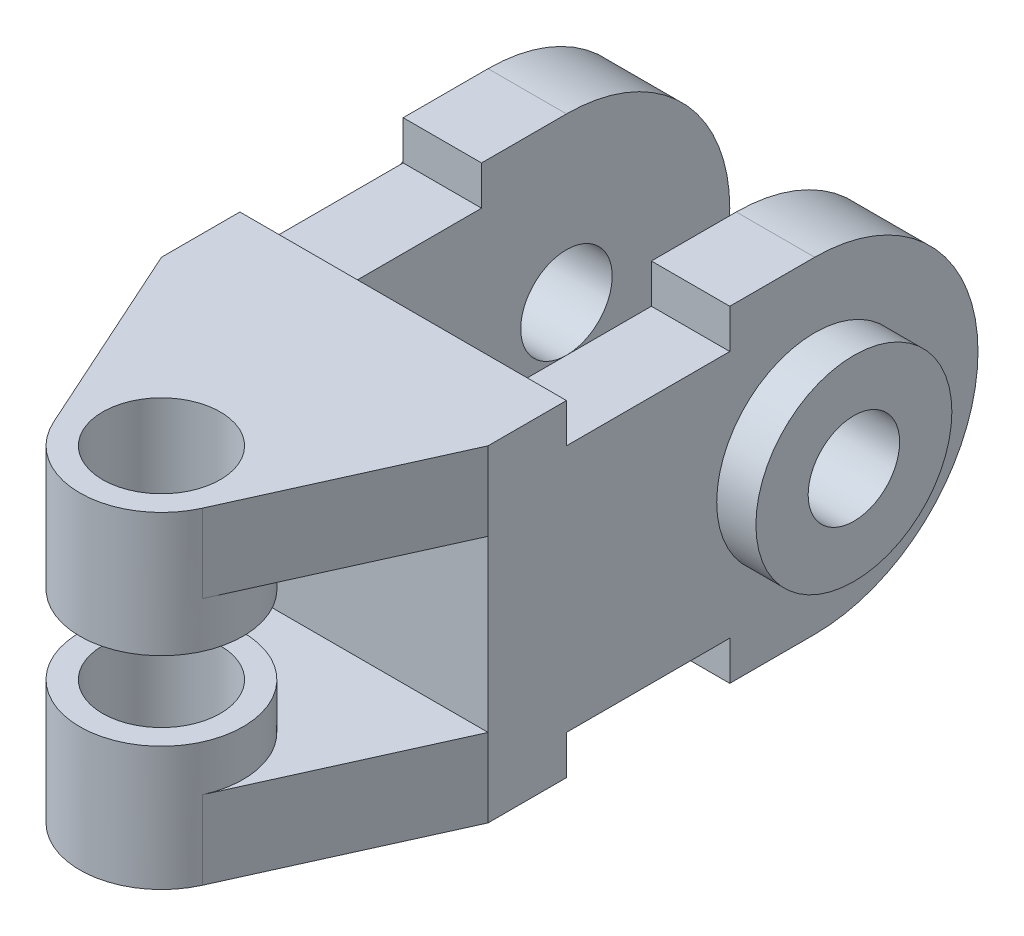
ISO-10303-21;
HEADER;
FILE_DESCRIPTION(('STEP AP214'),'2;1');
FILE_NAME('part.step','',(''),(''),'','','');
FILE_SCHEMA(('AUTOMOTIVE_DESIGN { 1 0 10303 214 1 1 1 1 }'));
ENDSEC;
DATA;
#1=APPLICATION_CONTEXT('core data for automotive mechanical design processes');
#2=APPLICATION_PROTOCOL_DEFINITION('international standard','automotive_design',2000,#1);
#3=PRODUCT_CONTEXT('',#1,'mechanical');
#4=PRODUCT('Part','Part','',(#3));
#5=PRODUCT_RELATED_PRODUCT_CATEGORY('part','',(#4));
#6=PRODUCT_DEFINITION_FORMATION('','',#4);
#7=PRODUCT_DEFINITION_CONTEXT('part definition',#1,'design');
#8=PRODUCT_DEFINITION('design','',#6,#7);
#9=PRODUCT_DEFINITION_SHAPE('','',#8);
#10=(LENGTH_UNIT() NAMED_UNIT(*) SI_UNIT(.MILLI.,.METRE.));
#11=(NAMED_UNIT(*) PLANE_ANGLE_UNIT() SI_UNIT($,.RADIAN.));
#12=(NAMED_UNIT(*) SI_UNIT($,.STERADIAN.) SOLID_ANGLE_UNIT());
#13=UNCERTAINTY_MEASURE_WITH_UNIT(LENGTH_MEASURE(1.E-05),#10,'distance_accuracy_value','');
#14=(GEOMETRIC_REPRESENTATION_CONTEXT(3) GLOBAL_UNCERTAINTY_ASSIGNED_CONTEXT((#13)) GLOBAL_UNIT_ASSIGNED_CONTEXT((#10,
#11,#12)) REPRESENTATION_CONTEXT('',''));
#15=CARTESIAN_POINT('',(0.,0.,0.));
#16=DIRECTION('',(0.,0.,1.));
#17=DIRECTION('',(1.,0.,0.));
#18=AXIS2_PLACEMENT_3D('',#15,#16,#17);
#19=CARTESIAN_POINT('',(0.,12.,0.));
#20=DIRECTION('',(0.,-1.,0.));
#21=DIRECTION('',(0.,0.,-1.));
#22=AXIS2_PLACEMENT_3D('',#19,#20,#21);
#23=PLANE('',#22);
#24=CARTESIAN_POINT('',(-13.,12.,25.));
#25=DIRECTION('',(0.,1.,0.));
#26=DIRECTION('',(0.,0.,1.));
#27=AXIS2_PLACEMENT_3D('',#24,#25,#26);
#28=CIRCLE('',#27,12.5);
#29=CARTESIAN_POINT('',(-1.60702715292317,12.,30.1429728470769));
#30=VERTEX_POINT('',#29);
#31=CARTESIAN_POINT('',(-24.3929728470769,12.,30.1429728470769));
#32=VERTEX_POINT('',#31);
#33=EDGE_CURVE('E226',#30,#32,#28,.T.);
#34=ORIENTED_EDGE('',*,*,#33,.F.);
#35=DIRECTION('',(0.411437827766148,0.,-0.911437827766148));
#36=VECTOR('',#35,1.);
#37=CARTESIAN_POINT('',(9.96862696659688,12.,4.5));
#38=LINE('',#37,#36);
#39=CARTESIAN_POINT('',(12.,12.,0.));
#40=VERTEX_POINT('',#39);
#41=EDGE_CURVE('E234',#30,#40,#38,.T.);
#42=ORIENTED_EDGE('',*,*,#41,.T.);
#43=DIRECTION('',(-1.,0.,0.));
#44=VECTOR('',#43,1.);
#45=CARTESIAN_POINT('',(0.,12.,0.));
#46=LINE('',#45,#44);
#47=CARTESIAN_POINT('',(-38.,12.,0.));
#48=VERTEX_POINT('',#47);
#49=EDGE_CURVE('E233',#40,#48,#46,.T.);
#50=ORIENTED_EDGE('',*,*,#49,.T.);
#51=DIRECTION('',(0.411437827766148,0.,0.911437827766148));
#52=VECTOR('',#51,1.);
#53=CARTESIAN_POINT('',(-31.5673187275568,12.,14.25));
#54=LINE('',#53,#52);
#55=EDGE_CURVE('E217',#48,#32,#54,.T.);
#56=ORIENTED_EDGE('',*,*,#55,.T.);
#57=EDGE_LOOP('',(#34,#42,#50,#56));
#58=FACE_BOUND('',#57,.T.);
#59=ADVANCED_FACE('F41',(#58),#23,.F.);
#60=CARTESIAN_POINT('',(12.,0.,0.));
#61=DIRECTION('',(0.,0.,-1.));
#62=DIRECTION('',(-1.,0.,0.));
#63=AXIS2_PLACEMENT_3D('',#60,#61,#62);
#64=PLANE('',#63);
#65=ORIENTED_EDGE('',*,*,#49,.F.);
#66=DIRECTION('',(0.,-1.,0.));
#67=VECTOR('',#66,1.);
#68=CARTESIAN_POINT('',(12.,0.,0.));
#69=LINE('',#68,#67);
#70=CARTESIAN_POINT('',(12.,38.,0.));
#71=VERTEX_POINT('',#70);
#72=EDGE_CURVE('E403',#71,#40,#69,.T.);
#73=ORIENTED_EDGE('',*,*,#72,.F.);
#74=DIRECTION('',(-1.,0.,0.));
#75=VECTOR('',#74,1.);
#76=CARTESIAN_POINT('',(-38.,38.,0.));
#77=LINE('',#76,#75);
#78=CARTESIAN_POINT('',(-38.,38.,0.));
#79=VERTEX_POINT('',#78);
#80=EDGE_CURVE('E267',#71,#79,#77,.T.);
#81=ORIENTED_EDGE('',*,*,#80,.T.);
#82=DIRECTION('',(0.,-1.,0.));
#83=VECTOR('',#82,1.);
#84=CARTESIAN_POINT('',(-38.,50.,0.));
#85=LINE('',#84,#83);
#86=EDGE_CURVE('E355',#79,#48,#85,.T.);
#87=ORIENTED_EDGE('',*,*,#86,.T.);
#88=EDGE_LOOP('',(#65,#73,#81,#87));
#89=FACE_BOUND('',#88,.T.);
#90=ADVANCED_FACE('F481',(#89),#64,.F.);
#91=CARTESIAN_POINT('',(-38.,50.,-12.));
#92=DIRECTION('',(-1.,0.,0.));
#93=DIRECTION('',(0.,0.,1.));
#94=AXIS2_PLACEMENT_3D('',#91,#92,#93);
#95=PLANE('',#94);
#96=CARTESIAN_POINT('',(-38.,50.,0.));
#97=VERTEX_POINT('',#96);
#98=EDGE_CURVE('E375',#97,#79,#85,.T.);
#99=ORIENTED_EDGE('',*,*,#98,.F.);
#100=DIRECTION('',(0.,0.,1.));
#101=VECTOR('',#100,1.);
#102=CARTESIAN_POINT('',(-38.,50.,-12.));
#103=LINE('',#102,#101);
#104=CARTESIAN_POINT('',(-38.,50.,-12.));
#105=VERTEX_POINT('',#104);
#106=EDGE_CURVE('E367',#105,#97,#103,.T.);
#107=ORIENTED_EDGE('',*,*,#106,.F.);
#108=DIRECTION('',(0.,-1.,0.));
#109=VECTOR('',#108,1.);
#110=CARTESIAN_POINT('',(-38.,50.,-12.));
#111=LINE('',#110,#109);
#112=CARTESIAN_POINT('',(-38.,44.,-12.));
#113=VERTEX_POINT('',#112);
#114=EDGE_CURVE('E370',#105,#113,#111,.T.);
#115=ORIENTED_EDGE('',*,*,#114,.T.);
#116=DIRECTION('',(0.,0.,-1.));
#117=VECTOR('',#116,1.);
#118=CARTESIAN_POINT('',(-38.,44.,-12.));
#119=LINE('',#118,#117);
#120=CARTESIAN_POINT('',(-38.,44.,-37.));
#121=VERTEX_POINT('',#120);
#122=EDGE_CURVE('E307',#113,#121,#119,.T.);
#123=ORIENTED_EDGE('',*,*,#122,.T.);
#124=DIRECTION('',(0.,1.,0.));
#125=VECTOR('',#124,1.);
#126=CARTESIAN_POINT('',(-38.,44.,-37.));
#127=LINE('',#126,#125);
#128=CARTESIAN_POINT('',(-38.,50.,-37.));
#129=VERTEX_POINT('',#128);
#130=EDGE_CURVE('E333',#121,#129,#127,.T.);
#131=ORIENTED_EDGE('',*,*,#130,.T.);
#132=DIRECTION('',(0.,0.,-1.));
#133=VECTOR('',#132,1.);
#134=CARTESIAN_POINT('',(-38.,50.,-37.));
#135=LINE('',#134,#133);
#136=CARTESIAN_POINT('',(-38.,50.,-50.));
#137=VERTEX_POINT('',#136);
#138=EDGE_CURVE('E338',#129,#137,#135,.T.);
#139=ORIENTED_EDGE('',*,*,#138,.T.);
#140=CARTESIAN_POINT('',(-38.,25.,-50.));
#141=DIRECTION('',(-1.,0.,0.));
#142=DIRECTION('',(0.,0.,1.));
#143=AXIS2_PLACEMENT_3D('',#140,#141,#142);
#144=CIRCLE('',#143,25.);
#145=CARTESIAN_POINT('',(-38.,0.,-50.));
#146=VERTEX_POINT('',#145);
#147=EDGE_CURVE('E342',#137,#146,#144,.T.);
#148=ORIENTED_EDGE('',*,*,#147,.T.);
#149=DIRECTION('',(0.,0.,1.));
#150=VECTOR('',#149,1.);
#151=CARTESIAN_POINT('',(-38.,0.,-37.));
#152=LINE('',#151,#150);
#153=CARTESIAN_POINT('',(-38.,0.,-37.));
#154=VERTEX_POINT('',#153);
#155=EDGE_CURVE('E344',#146,#154,#152,.T.);
#156=ORIENTED_EDGE('',*,*,#155,.T.);
#157=DIRECTION('',(0.,1.,0.));
#158=VECTOR('',#157,1.);
#159=CARTESIAN_POINT('',(-38.,6.,-37.));
#160=LINE('',#159,#158);
#161=CARTESIAN_POINT('',(-38.,6.,-37.));
#162=VERTEX_POINT('',#161);
#163=EDGE_CURVE('E350',#154,#162,#160,.T.);
#164=ORIENTED_EDGE('',*,*,#163,.T.);
#165=DIRECTION('',(0.,0.,1.));
#166=VECTOR('',#165,1.);
#167=CARTESIAN_POINT('',(-38.,6.,-12.));
#168=LINE('',#167,#166);
#169=CARTESIAN_POINT('',(-38.,6.,-12.));
#170=VERTEX_POINT('',#169);
#171=EDGE_CURVE('E64',#162,#170,#168,.T.);
#172=ORIENTED_EDGE('',*,*,#171,.T.);
#173=CARTESIAN_POINT('',(-38.,0.,-12.));
#174=VERTEX_POINT('',#173);
#175=EDGE_CURVE('E371',#170,#174,#111,.T.);
#176=ORIENTED_EDGE('',*,*,#175,.T.);
#177=DIRECTION('',(0.,0.,1.));
#178=VECTOR('',#177,1.);
#179=CARTESIAN_POINT('',(-38.,0.,-12.));
#180=LINE('',#179,#178);
#181=CARTESIAN_POINT('',(-38.,0.,0.));
#182=VERTEX_POINT('',#181);
#183=EDGE_CURVE('E372',#174,#182,#180,.T.);
#184=ORIENTED_EDGE('',*,*,#183,.T.);
#185=DIRECTION('',(0.,-1.,0.));
#186=VECTOR('',#185,1.);
#187=CARTESIAN_POINT('',(-38.,12.,0.));
#188=LINE('',#187,#186);
#189=EDGE_CURVE('E227',#48,#182,#188,.T.);
#190=ORIENTED_EDGE('',*,*,#189,.F.);
#191=ORIENTED_EDGE('',*,*,#86,.F.);
#192=EDGE_LOOP('',(#99,#107,#115,#123,#131,#139,#148,#156,#164,#172,#176,#184,#190,#191));
#193=FACE_BOUND('',#192,.T.);
#194=CARTESIAN_POINT('',(-38.,25.,-50.));
#195=DIRECTION('',(-1.,0.,0.));
#196=DIRECTION('',(0.,0.,1.));
#197=AXIS2_PLACEMENT_3D('',#194,#195,#196);
#198=CIRCLE('',#197,15.);
#199=CARTESIAN_POINT('',(-38.,25.,-35.));
#200=VERTEX_POINT('',#199);
#201=EDGE_CURVE('E292',#200,#200,#198,.T.);
#202=ORIENTED_EDGE('',*,*,#201,.F.);
#203=EDGE_LOOP('',(#202));
#204=FACE_BOUND('',#203,.T.);
#205=ADVANCED_FACE('F488',(#193,#204),#95,.T.);
#206=CARTESIAN_POINT('',(12.,0.,-12.));
#207=DIRECTION('',(0.,1.,0.));
#208=DIRECTION('',(0.,0.,1.));
#209=AXIS2_PLACEMENT_3D('',#206,#207,#208);
#210=PLANE('',#209);
#211=DIRECTION('',(0.,0.,-1.));
#212=VECTOR('',#211,1.);
#213=CARTESIAN_POINT('',(12.,0.,-12.));
#214=LINE('',#213,#212);
#215=CARTESIAN_POINT('',(12.,0.,0.));
#216=VERTEX_POINT('',#215);
#217=CARTESIAN_POINT('',(12.,0.,-12.));
#218=VERTEX_POINT('',#217);
#219=EDGE_CURVE('E379',#216,#218,#214,.T.);
#220=ORIENTED_EDGE('',*,*,#219,.F.);
#221=DIRECTION('',(0.411437827766148,0.,-0.911437827766148));
#222=VECTOR('',#221,1.);
#223=CARTESIAN_POINT('',(9.96862696659688,0.,4.5));
#224=LINE('',#223,#222);
#225=CARTESIAN_POINT('',(-1.60702715292317,0.,30.1429728470769));
#226=VERTEX_POINT('',#225);
#227=EDGE_CURVE('E243',#226,#216,#224,.T.);
#228=ORIENTED_EDGE('',*,*,#227,.F.);
#229=CARTESIAN_POINT('',(-13.,0.,25.));
#230=DIRECTION('',(0.,-1.,0.));
#231=DIRECTION('',(0.,0.,-1.));
#232=AXIS2_PLACEMENT_3D('',#229,#230,#231);
#233=CIRCLE('',#232,12.5);
#234=CARTESIAN_POINT('',(-24.3929728470768,0.,30.1429728470769));
#235=VERTEX_POINT('',#234);
#236=EDGE_CURVE('E252',#226,#235,#233,.T.);
#237=ORIENTED_EDGE('',*,*,#236,.T.);
#238=DIRECTION('',(0.411437827766148,0.,0.911437827766148));
#239=VECTOR('',#238,1.);
#240=CARTESIAN_POINT('',(-31.5673187275568,0.,14.25));
#241=LINE('',#240,#239);
#242=EDGE_CURVE('E222',#182,#235,#241,.T.);
#243=ORIENTED_EDGE('',*,*,#242,.F.);
#244=ORIENTED_EDGE('',*,*,#183,.F.);
#245=DIRECTION('',(-1.,0.,0.));
#246=VECTOR('',#245,1.);
#247=CARTESIAN_POINT('',(12.,0.,-12.));
#248=LINE('',#247,#246);
#249=EDGE_CURVE('E448',#218,#174,#248,.T.);
#250=ORIENTED_EDGE('',*,*,#249,.F.);
#251=EDGE_LOOP('',(#220,#228,#237,#243,#244,#250));
#252=FACE_BOUND('',#251,.T.);
#253=CARTESIAN_POINT('',(-13.,0.,25.));
#254=DIRECTION('',(0.,-1.,0.));
#255=DIRECTION('',(0.,0.,-1.));
#256=AXIS2_PLACEMENT_3D('',#253,#254,#255);
#257=CIRCLE('',#256,9.);
#258=CARTESIAN_POINT('',(-13.,0.,16.));
#259=VERTEX_POINT('',#258);
#260=EDGE_CURVE('E248',#259,#259,#257,.T.);
#261=ORIENTED_EDGE('',*,*,#260,.F.);
#262=EDGE_LOOP('',(#261));
#263=FACE_BOUND('',#262,.T.);
#264=ADVANCED_FACE('F43',(#252,#263),#210,.F.);
#265=CARTESIAN_POINT('',(12.,6.,-37.));
#266=DIRECTION('',(0.,1.,0.));
#267=DIRECTION('',(0.,0.,1.));
#268=AXIS2_PLACEMENT_3D('',#265,#266,#267);
#269=PLANE('',#268);
#270=DIRECTION('',(0.,0.,-1.));
#271=VECTOR('',#270,1.);
#272=CARTESIAN_POINT('',(0.,6.,-37.));
#273=LINE('',#272,#271);
#274=CARTESIAN_POINT('',(0.,6.,-12.));
#275=VERTEX_POINT('',#274);
#276=CARTESIAN_POINT('',(0.,6.,-37.));
#277=VERTEX_POINT('',#276);
#278=EDGE_CURVE('E380',#275,#277,#273,.T.);
#279=ORIENTED_EDGE('',*,*,#278,.T.);
#280=DIRECTION('',(-1.,0.,0.));
#281=VECTOR('',#280,1.);
#282=CARTESIAN_POINT('',(12.,6.,-37.));
#283=LINE('',#282,#281);
#284=CARTESIAN_POINT('',(12.,6.,-37.));
#285=VERTEX_POINT('',#284);
#286=EDGE_CURVE('E445',#285,#277,#283,.T.);
#287=ORIENTED_EDGE('',*,*,#286,.F.);
#288=DIRECTION('',(0.,0.,-1.));
#289=VECTOR('',#288,1.);
#290=CARTESIAN_POINT('',(12.,6.,-37.));
#291=LINE('',#290,#289);
#292=CARTESIAN_POINT('',(12.,6.,-12.));
#293=VERTEX_POINT('',#292);
#294=EDGE_CURVE('E387',#293,#285,#291,.T.);
#295=ORIENTED_EDGE('',*,*,#294,.F.);
#296=DIRECTION('',(-1.,0.,0.));
#297=VECTOR('',#296,1.);
#298=CARTESIAN_POINT('',(12.,6.,-12.));
#299=LINE('',#298,#297);
#300=EDGE_CURVE('E443',#293,#275,#299,.T.);
#301=ORIENTED_EDGE('',*,*,#300,.T.);
#302=EDGE_LOOP('',(#279,#287,#295,#301));
#303=FACE_BOUND('',#302,.T.);
#304=ADVANCED_FACE('F591',(#303),#269,.F.);
#305=CARTESIAN_POINT('',(12.,0.,-37.));
#306=DIRECTION('',(0.,0.,-1.));
#307=DIRECTION('',(-1.,0.,0.));
#308=AXIS2_PLACEMENT_3D('',#305,#306,#307);
#309=PLANE('',#308);
#310=DIRECTION('',(0.,-1.,0.));
#311=VECTOR('',#310,1.);
#312=CARTESIAN_POINT('',(0.,0.,-37.));
#313=LINE('',#312,#311);
#314=CARTESIAN_POINT('',(0.,0.,-37.));
#315=VERTEX_POINT('',#314);
#316=EDGE_CURVE('E412',#277,#315,#313,.T.);
#317=ORIENTED_EDGE('',*,*,#316,.T.);
#318=DIRECTION('',(-1.,0.,0.));
#319=VECTOR('',#318,1.);
#320=CARTESIAN_POINT('',(12.,0.,-37.));
#321=LINE('',#320,#319);
#322=CARTESIAN_POINT('',(12.,0.,-37.));
#323=VERTEX_POINT('',#322);
#324=EDGE_CURVE('E438',#323,#315,#321,.T.);
#325=ORIENTED_EDGE('',*,*,#324,.F.);
#326=DIRECTION('',(0.,-1.,0.));
#327=VECTOR('',#326,1.);
#328=CARTESIAN_POINT('',(12.,0.,-37.));
#329=LINE('',#328,#327);
#330=EDGE_CURVE('E389',#285,#323,#329,.T.);
#331=ORIENTED_EDGE('',*,*,#330,.F.);
#332=ORIENTED_EDGE('',*,*,#286,.T.);
#333=EDGE_LOOP('',(#317,#325,#331,#332));
#334=FACE_BOUND('',#333,.T.);
#335=ADVANCED_FACE('F596',(#334),#309,.F.);
#336=CARTESIAN_POINT('',(12.,0.,-50.));
#337=DIRECTION('',(0.,1.,0.));
#338=DIRECTION('',(0.,0.,1.));
#339=AXIS2_PLACEMENT_3D('',#336,#337,#338);
#340=PLANE('',#339);
#341=DIRECTION('',(0.,0.,-1.));
#342=VECTOR('',#341,1.);
#343=CARTESIAN_POINT('',(0.,0.,-50.));
#344=LINE('',#343,#342);
#345=CARTESIAN_POINT('',(0.,0.,-50.));
#346=VERTEX_POINT('',#345);
#347=EDGE_CURVE('E413',#315,#346,#344,.T.);
#348=ORIENTED_EDGE('',*,*,#347,.T.);
#349=DIRECTION('',(-1.,0.,0.));
#350=VECTOR('',#349,1.);
#351=CARTESIAN_POINT('',(12.,0.,-50.));
#352=LINE('',#351,#350);
#353=CARTESIAN_POINT('',(12.,0.,-50.));
#354=VERTEX_POINT('',#353);
#355=EDGE_CURVE('E436',#354,#346,#352,.T.);
#356=ORIENTED_EDGE('',*,*,#355,.F.);
#357=DIRECTION('',(0.,0.,-1.));
#358=VECTOR('',#357,1.);
#359=CARTESIAN_POINT('',(12.,0.,-50.));
#360=LINE('',#359,#358);
#361=EDGE_CURVE('E388',#323,#354,#360,.T.);
#362=ORIENTED_EDGE('',*,*,#361,.F.);
#363=ORIENTED_EDGE('',*,*,#324,.T.);
#364=EDGE_LOOP('',(#348,#356,#362,#363));
#365=FACE_BOUND('',#364,.T.);
#366=ADVANCED_FACE('F605',(#365),#340,.F.);
#367=CARTESIAN_POINT('',(12.,25.,-50.));
#368=DIRECTION('',(-1.,0.,0.));
#369=DIRECTION('',(0.,0.,1.));
#370=AXIS2_PLACEMENT_3D('',#367,#368,#369);
#371=CYLINDRICAL_SURFACE('',#370,25.);
#372=CARTESIAN_POINT('',(0.,25.,-50.));
#373=DIRECTION('',(1.,0.,0.));
#374=DIRECTION('',(0.,0.,1.));
#375=AXIS2_PLACEMENT_3D('',#372,#373,#374);
#376=CIRCLE('',#375,25.);
#377=CARTESIAN_POINT('',(0.,50.,-50.));
#378=VERTEX_POINT('',#377);
#379=EDGE_CURVE('E411',#346,#378,#376,.T.);
#380=ORIENTED_EDGE('',*,*,#379,.T.);
#381=DIRECTION('',(-1.,0.,0.));
#382=VECTOR('',#381,1.);
#383=CARTESIAN_POINT('',(12.,50.,-50.));
#384=LINE('',#383,#382);
#385=CARTESIAN_POINT('',(12.,50.,-50.));
#386=VERTEX_POINT('',#385);
#387=EDGE_CURVE('E433',#386,#378,#384,.T.);
#388=ORIENTED_EDGE('',*,*,#387,.F.);
#389=CARTESIAN_POINT('',(12.,25.,-50.));
#390=DIRECTION('',(1.,0.,0.));
#391=DIRECTION('',(0.,0.,1.));
#392=AXIS2_PLACEMENT_3D('',#389,#390,#391);
#393=CIRCLE('',#392,25.);
#394=EDGE_CURVE('E395',#354,#386,#393,.T.);
#395=ORIENTED_EDGE('',*,*,#394,.F.);
#396=ORIENTED_EDGE('',*,*,#355,.T.);
#397=EDGE_LOOP('',(#380,#388,#395,#396));
#398=FACE_BOUND('',#397,.T.);
#399=ADVANCED_FACE('F607',(#398),#371,.T.);
#400=CARTESIAN_POINT('',(12.,50.,-37.));
#401=DIRECTION('',(0.,-1.,0.));
#402=DIRECTION('',(0.,0.,-1.));
#403=AXIS2_PLACEMENT_3D('',#400,#401,#402);
#404=PLANE('',#403);
#405=DIRECTION('',(0.,0.,1.));
#406=VECTOR('',#405,1.);
#407=CARTESIAN_POINT('',(0.,50.,-37.));
#408=LINE('',#407,#406);
#409=CARTESIAN_POINT('',(0.,50.,-37.));
#410=VERTEX_POINT('',#409);
#411=EDGE_CURVE('E417',#378,#410,#408,.T.);
#412=ORIENTED_EDGE('',*,*,#411,.T.);
#413=DIRECTION('',(-1.,0.,0.));
#414=VECTOR('',#413,1.);
#415=CARTESIAN_POINT('',(12.,50.,-37.));
#416=LINE('',#415,#414);
#417=CARTESIAN_POINT('',(12.,50.,-37.));
#418=VERTEX_POINT('',#417);
#419=EDGE_CURVE('E429',#418,#410,#416,.T.);
#420=ORIENTED_EDGE('',*,*,#419,.F.);
#421=DIRECTION('',(0.,0.,1.));
#422=VECTOR('',#421,1.);
#423=CARTESIAN_POINT('',(12.,50.,-37.));
#424=LINE('',#423,#422);
#425=EDGE_CURVE('E394',#386,#418,#424,.T.);
#426=ORIENTED_EDGE('',*,*,#425,.F.);
#427=ORIENTED_EDGE('',*,*,#387,.T.);
#428=EDGE_LOOP('',(#412,#420,#426,#427));
#429=FACE_BOUND('',#428,.T.);
#430=ADVANCED_FACE('F612',(#429),#404,.F.);
#431=CARTESIAN_POINT('',(12.,44.,-37.));
#432=DIRECTION('',(0.,0.,-1.));
#433=DIRECTION('',(-1.,0.,0.));
#434=AXIS2_PLACEMENT_3D('',#431,#432,#433);
#435=PLANE('',#434);
#436=DIRECTION('',(0.,-1.,0.));
#437=VECTOR('',#436,1.);
#438=CARTESIAN_POINT('',(0.,44.,-37.));
#439=LINE('',#438,#437);
#440=CARTESIAN_POINT('',(0.,44.,-37.));
#441=VERTEX_POINT('',#440);
#442=EDGE_CURVE('E420',#410,#441,#439,.T.);
#443=ORIENTED_EDGE('',*,*,#442,.T.);
#444=DIRECTION('',(-1.,0.,0.));
#445=VECTOR('',#444,1.);
#446=CARTESIAN_POINT('',(12.,44.,-37.));
#447=LINE('',#446,#445);
#448=CARTESIAN_POINT('',(12.,44.,-37.));
#449=VERTEX_POINT('',#448);
#450=EDGE_CURVE('E430',#449,#441,#447,.T.);
#451=ORIENTED_EDGE('',*,*,#450,.F.);
#452=DIRECTION('',(0.,-1.,0.));
#453=VECTOR('',#452,1.);
#454=CARTESIAN_POINT('',(12.,44.,-37.));
#455=LINE('',#454,#453);
#456=EDGE_CURVE('E397',#418,#449,#455,.T.);
#457=ORIENTED_EDGE('',*,*,#456,.F.);
#458=ORIENTED_EDGE('',*,*,#419,.T.);
#459=EDGE_LOOP('',(#443,#451,#457,#458));
#460=FACE_BOUND('',#459,.T.);
#461=ADVANCED_FACE('F611',(#460),#435,.F.);
#462=CARTESIAN_POINT('',(12.,44.,-12.));
#463=DIRECTION('',(0.,-1.,0.));
#464=DIRECTION('',(0.,0.,-1.));
#465=AXIS2_PLACEMENT_3D('',#462,#463,#464);
#466=PLANE('',#465);
#467=DIRECTION('',(0.,0.,1.));
#468=VECTOR('',#467,1.);
#469=CARTESIAN_POINT('',(0.,44.,-12.));
#470=LINE('',#469,#468);
#471=CARTESIAN_POINT('',(0.,44.,-12.));
#472=VERTEX_POINT('',#471);
#473=EDGE_CURVE('E383',#441,#472,#470,.T.);
#474=ORIENTED_EDGE('',*,*,#473,.T.);
#475=DIRECTION('',(-1.,0.,0.));
#476=VECTOR('',#475,1.);
#477=CARTESIAN_POINT('',(12.,44.,-12.));
#478=LINE('',#477,#476);
#479=CARTESIAN_POINT('',(12.,44.,-12.));
#480=VERTEX_POINT('',#479);
#481=EDGE_CURVE('E424',#480,#472,#478,.T.);
#482=ORIENTED_EDGE('',*,*,#481,.F.);
#483=DIRECTION('',(0.,0.,1.));
#484=VECTOR('',#483,1.);
#485=CARTESIAN_POINT('',(12.,44.,-12.));
#486=LINE('',#485,#484);
#487=EDGE_CURVE('E398',#449,#480,#486,.T.);
#488=ORIENTED_EDGE('',*,*,#487,.F.);
#489=ORIENTED_EDGE('',*,*,#450,.T.);
#490=EDGE_LOOP('',(#474,#482,#488,#489));
#491=FACE_BOUND('',#490,.T.);
#492=ADVANCED_FACE('F619',(#491),#466,.F.);
#493=CARTESIAN_POINT('',(12.,50.,-12.));
#494=DIRECTION('',(0.,0.,1.));
#495=DIRECTION('',(1.,0.,0.));
#496=AXIS2_PLACEMENT_3D('',#493,#494,#495);
#497=PLANE('',#496);
#498=ORIENTED_EDGE('',*,*,#175,.F.);
#499=DIRECTION('',(-1.,0.,0.));
#500=VECTOR('',#499,1.);
#501=CARTESIAN_POINT('',(-26.,6.,-12.));
#502=LINE('',#501,#500);
#503=CARTESIAN_POINT('',(-26.,6.,-12.));
#504=VERTEX_POINT('',#503);
#505=EDGE_CURVE('E348',#504,#170,#502,.T.);
#506=ORIENTED_EDGE('',*,*,#505,.F.);
#507=DIRECTION('',(0.,1.,0.));
#508=VECTOR('',#507,1.);
#509=CARTESIAN_POINT('',(-26.,44.,-12.));
#510=LINE('',#509,#508);
#511=CARTESIAN_POINT('',(-26.,44.,-12.));
#512=VERTEX_POINT('',#511);
#513=EDGE_CURVE('E306',#504,#512,#510,.T.);
#514=ORIENTED_EDGE('',*,*,#513,.T.);
#515=DIRECTION('',(-1.,0.,0.));
#516=VECTOR('',#515,1.);
#517=CARTESIAN_POINT('',(-26.,44.,-12.));
#518=LINE('',#517,#516);
#519=EDGE_CURVE('E335',#512,#113,#518,.T.);
#520=ORIENTED_EDGE('',*,*,#519,.T.);
#521=ORIENTED_EDGE('',*,*,#114,.F.);
#522=DIRECTION('',(-1.,0.,0.));
#523=VECTOR('',#522,1.);
#524=CARTESIAN_POINT('',(12.,50.,-12.));
#525=LINE('',#524,#523);
#526=CARTESIAN_POINT('',(12.,50.,-12.));
#527=VERTEX_POINT('',#526);
#528=EDGE_CURVE('E409',#527,#105,#525,.T.);
#529=ORIENTED_EDGE('',*,*,#528,.F.);
#530=DIRECTION('',(0.,1.,0.));
#531=VECTOR('',#530,1.);
#532=CARTESIAN_POINT('',(12.,50.,-12.));
#533=LINE('',#532,#531);
#534=EDGE_CURVE('E396',#480,#527,#533,.T.);
#535=ORIENTED_EDGE('',*,*,#534,.F.);
#536=ORIENTED_EDGE('',*,*,#481,.T.);
#537=DIRECTION('',(0.,-1.,0.));
#538=VECTOR('',#537,1.);
#539=CARTESIAN_POINT('',(0.,25.,-12.));
#540=LINE('',#539,#538);
#541=EDGE_CURVE('E452',#472,#275,#540,.T.);
#542=ORIENTED_EDGE('',*,*,#541,.T.);
#543=ORIENTED_EDGE('',*,*,#300,.F.);
#544=DIRECTION('',(0.,1.,0.));
#545=VECTOR('',#544,1.);
#546=CARTESIAN_POINT('',(12.,6.,-12.));
#547=LINE('',#546,#545);
#548=EDGE_CURVE('E382',#218,#293,#547,.T.);
#549=ORIENTED_EDGE('',*,*,#548,.F.);
#550=ORIENTED_EDGE('',*,*,#249,.T.);
#551=EDGE_LOOP('',(#498,#506,#514,#520,#521,#529,#535,#536,#542,#543,#549,#550));
#552=FACE_BOUND('',#551,.T.);
#553=ADVANCED_FACE('F552',(#552),#497,.F.);
#554=CARTESIAN_POINT('',(12.,50.,0.));
#555=DIRECTION('',(0.,-1.,0.));
#556=DIRECTION('',(0.,0.,-1.));
#557=AXIS2_PLACEMENT_3D('',#554,#555,#556);
#558=PLANE('',#557);
#559=CARTESIAN_POINT('',(-13.,50.,25.));
#560=DIRECTION('',(0.,1.,0.));
#561=DIRECTION('',(0.,0.,1.));
#562=AXIS2_PLACEMENT_3D('',#559,#560,#561);
#563=CIRCLE('',#562,9.);
#564=CARTESIAN_POINT('',(-13.,50.,34.));
#565=VERTEX_POINT('',#564);
#566=EDGE_CURVE('E257',#565,#565,#563,.T.);
#567=ORIENTED_EDGE('',*,*,#566,.F.);
#568=EDGE_LOOP('',(#567));
#569=FACE_BOUND('',#568,.T.);
#570=DIRECTION('',(0.411437827766148,0.,0.911437827766148));
#571=VECTOR('',#570,1.);
#572=CARTESIAN_POINT('',(-38.,50.,0.));
#573=LINE('',#572,#571);
#574=CARTESIAN_POINT('',(-24.3929728470768,50.,30.1429728470768));
#575=VERTEX_POINT('',#574);
#576=EDGE_CURVE('E268',#97,#575,#573,.T.);
#577=ORIENTED_EDGE('',*,*,#576,.T.);
#578=CARTESIAN_POINT('',(-13.,50.,25.));
#579=DIRECTION('',(0.,1.,0.));
#580=DIRECTION('',(0.,0.,1.));
#581=AXIS2_PLACEMENT_3D('',#578,#579,#580);
#582=CIRCLE('',#581,12.5);
#583=CARTESIAN_POINT('',(-1.60702715292317,50.,30.1429728470768));
#584=VERTEX_POINT('',#583);
#585=EDGE_CURVE('E278',#575,#584,#582,.T.);
#586=ORIENTED_EDGE('',*,*,#585,.T.);
#587=DIRECTION('',(0.411437827766148,0.,-0.911437827766148));
#588=VECTOR('',#587,1.);
#589=CARTESIAN_POINT('',(-1.60702715292316,50.,30.1429728470768));
#590=LINE('',#589,#588);
#591=CARTESIAN_POINT('',(12.,50.,0.));
#592=VERTEX_POINT('',#591);
#593=EDGE_CURVE('E275',#584,#592,#590,.T.);
#594=ORIENTED_EDGE('',*,*,#593,.T.);
#595=DIRECTION('',(0.,0.,1.));
#596=VECTOR('',#595,1.);
#597=CARTESIAN_POINT('',(12.,50.,0.));
#598=LINE('',#597,#596);
#599=EDGE_CURVE('E405',#527,#592,#598,.T.);
#600=ORIENTED_EDGE('',*,*,#599,.F.);
#601=ORIENTED_EDGE('',*,*,#528,.T.);
#602=ORIENTED_EDGE('',*,*,#106,.T.);
#603=EDGE_LOOP('',(#577,#586,#594,#600,#601,#602));
#604=FACE_BOUND('',#603,.T.);
#605=ADVANCED_FACE('F533',(#569,#604),#558,.F.);
#606=CARTESIAN_POINT('',(12.,25.,-50.));
#607=DIRECTION('',(-1.,0.,0.));
#608=DIRECTION('',(0.,0.,1.));
#609=AXIS2_PLACEMENT_3D('',#606,#607,#608);
#610=PLANE('',#609);
#611=CARTESIAN_POINT('',(12.,25.,-50.));
#612=DIRECTION('',(-1.,0.,0.));
#613=DIRECTION('',(0.,0.,1.));
#614=AXIS2_PLACEMENT_3D('',#611,#612,#613);
#615=CIRCLE('',#614,15.);
#616=CARTESIAN_POINT('',(12.,25.,-35.));
#617=VERTEX_POINT('',#616);
#618=EDGE_CURVE('E49',#617,#617,#615,.F.);
#619=ORIENTED_EDGE('',*,*,#618,.F.);
#620=EDGE_LOOP('',(#619));
#621=FACE_BOUND('',#620,.T.);
#622=ORIENTED_EDGE('',*,*,#487,.T.);
#623=ORIENTED_EDGE('',*,*,#534,.T.);
#624=ORIENTED_EDGE('',*,*,#599,.T.);
#625=EDGE_CURVE('E407',#592,#71,#69,.T.);
#626=ORIENTED_EDGE('',*,*,#625,.T.);
#627=ORIENTED_EDGE('',*,*,#72,.T.);
#628=DIRECTION('',(0.,-1.,0.));
#629=VECTOR('',#628,1.);
#630=CARTESIAN_POINT('',(12.,12.,0.));
#631=LINE('',#630,#629);
#632=EDGE_CURVE('E260',#40,#216,#631,.T.);
#633=ORIENTED_EDGE('',*,*,#632,.T.);
#634=ORIENTED_EDGE('',*,*,#219,.T.);
#635=ORIENTED_EDGE('',*,*,#548,.T.);
#636=ORIENTED_EDGE('',*,*,#294,.T.);
#637=ORIENTED_EDGE('',*,*,#330,.T.);
#638=ORIENTED_EDGE('',*,*,#361,.T.);
#639=ORIENTED_EDGE('',*,*,#394,.T.);
#640=ORIENTED_EDGE('',*,*,#425,.T.);
#641=ORIENTED_EDGE('',*,*,#456,.T.);
#642=EDGE_LOOP('',(#622,#623,#624,#626,#627,#633,#634,#635,#636,#637,#638,#639,#640,#641));
#643=FACE_BOUND('',#642,.T.);
#644=ADVANCED_FACE('F544',(#621,#643),#610,.F.);
#645=CARTESIAN_POINT('',(0.,25.,-50.));
#646=DIRECTION('',(-1.,0.,0.));
#647=DIRECTION('',(0.,0.,1.));
#648=AXIS2_PLACEMENT_3D('',#645,#646,#647);
#649=PLANE('',#648);
#650=CARTESIAN_POINT('',(0.,25.,-50.));
#651=DIRECTION('',(-1.,0.,0.));
#652=DIRECTION('',(0.,0.,1.));
#653=AXIS2_PLACEMENT_3D('',#650,#651,#652);
#654=CIRCLE('',#653,7.);
#655=CARTESIAN_POINT('',(0.,25.,-43.));
#656=VERTEX_POINT('',#655);
#657=EDGE_CURVE('E298',#656,#656,#654,.T.);
#658=ORIENTED_EDGE('',*,*,#657,.F.);
#659=EDGE_LOOP('',(#658));
#660=FACE_BOUND('',#659,.T.);
#661=ORIENTED_EDGE('',*,*,#541,.F.);
#662=ORIENTED_EDGE('',*,*,#473,.F.);
#663=ORIENTED_EDGE('',*,*,#442,.F.);
#664=ORIENTED_EDGE('',*,*,#411,.F.);
#665=ORIENTED_EDGE('',*,*,#379,.F.);
#666=ORIENTED_EDGE('',*,*,#347,.F.);
#667=ORIENTED_EDGE('',*,*,#316,.F.);
#668=ORIENTED_EDGE('',*,*,#278,.F.);
#669=EDGE_LOOP('',(#661,#662,#663,#664,#665,#666,#667,#668));
#670=FACE_BOUND('',#669,.T.);
#671=ADVANCED_FACE('F622',(#660,#670),#649,.T.);
#672=CARTESIAN_POINT('',(-26.,6.,-12.));
#673=DIRECTION('',(0.,-1.,0.));
#674=DIRECTION('',(0.,0.,-1.));
#675=AXIS2_PLACEMENT_3D('',#672,#673,#674);
#676=PLANE('',#675);
#677=ORIENTED_EDGE('',*,*,#171,.F.);
#678=DIRECTION('',(-1.,0.,0.));
#679=VECTOR('',#678,1.);
#680=CARTESIAN_POINT('',(-26.,6.,-37.));
#681=LINE('',#680,#679);
#682=CARTESIAN_POINT('',(-26.,6.,-37.));
#683=VERTEX_POINT('',#682);
#684=EDGE_CURVE('E353',#683,#162,#681,.T.);
#685=ORIENTED_EDGE('',*,*,#684,.F.);
#686=DIRECTION('',(0.,0.,1.));
#687=VECTOR('',#686,1.);
#688=CARTESIAN_POINT('',(-26.,6.,-12.));
#689=LINE('',#688,#687);
#690=EDGE_CURVE('E328',#683,#504,#689,.T.);
#691=ORIENTED_EDGE('',*,*,#690,.T.);
#692=ORIENTED_EDGE('',*,*,#505,.T.);
#693=EDGE_LOOP('',(#677,#685,#691,#692));
#694=FACE_BOUND('',#693,.T.);
#695=ADVANCED_FACE('F577',(#694),#676,.T.);
#696=CARTESIAN_POINT('',(-26.,6.,-37.));
#697=DIRECTION('',(0.,0.,1.));
#698=DIRECTION('',(1.,0.,0.));
#699=AXIS2_PLACEMENT_3D('',#696,#697,#698);
#700=PLANE('',#699);
#701=ORIENTED_EDGE('',*,*,#163,.F.);
#702=DIRECTION('',(-1.,0.,0.));
#703=VECTOR('',#702,1.);
#704=CARTESIAN_POINT('',(-26.,0.,-37.));
#705=LINE('',#704,#703);
#706=CARTESIAN_POINT('',(-26.,0.,-37.));
#707=VERTEX_POINT('',#706);
#708=EDGE_CURVE('E351',#707,#154,#705,.T.);
#709=ORIENTED_EDGE('',*,*,#708,.F.);
#710=DIRECTION('',(0.,1.,0.));
#711=VECTOR('',#710,1.);
#712=CARTESIAN_POINT('',(-26.,6.,-37.));
#713=LINE('',#712,#711);
#714=EDGE_CURVE('E326',#707,#683,#713,.T.);
#715=ORIENTED_EDGE('',*,*,#714,.T.);
#716=ORIENTED_EDGE('',*,*,#684,.T.);
#717=EDGE_LOOP('',(#701,#709,#715,#716));
#718=FACE_BOUND('',#717,.T.);
#719=ADVANCED_FACE('F574',(#718),#700,.T.);
#720=CARTESIAN_POINT('',(-26.,0.,-37.));
#721=DIRECTION('',(0.,-1.,0.));
#722=DIRECTION('',(0.,0.,-1.));
#723=AXIS2_PLACEMENT_3D('',#720,#721,#722);
#724=PLANE('',#723);
#725=ORIENTED_EDGE('',*,*,#155,.F.);
#726=DIRECTION('',(-1.,0.,0.));
#727=VECTOR('',#726,1.);
#728=CARTESIAN_POINT('',(-26.,0.,-50.));
#729=LINE('',#728,#727);
#730=CARTESIAN_POINT('',(-26.,0.,-50.));
#731=VERTEX_POINT('',#730);
#732=EDGE_CURVE('E360',#731,#146,#729,.T.);
#733=ORIENTED_EDGE('',*,*,#732,.F.);
#734=DIRECTION('',(0.,0.,1.));
#735=VECTOR('',#734,1.);
#736=CARTESIAN_POINT('',(-26.,0.,-37.));
#737=LINE('',#736,#735);
#738=EDGE_CURVE('E323',#731,#707,#737,.T.);
#739=ORIENTED_EDGE('',*,*,#738,.T.);
#740=ORIENTED_EDGE('',*,*,#708,.T.);
#741=EDGE_LOOP('',(#725,#733,#739,#740));
#742=FACE_BOUND('',#741,.T.);
#743=ADVANCED_FACE('F568',(#742),#724,.T.);
#744=CARTESIAN_POINT('',(-26.,25.,-50.));
#745=DIRECTION('',(-1.,0.,0.));
#746=DIRECTION('',(0.,0.,1.));
#747=AXIS2_PLACEMENT_3D('',#744,#745,#746);
#748=CYLINDRICAL_SURFACE('',#747,25.);
#749=ORIENTED_EDGE('',*,*,#147,.F.);
#750=DIRECTION('',(-1.,0.,0.));
#751=VECTOR('',#750,1.);
#752=CARTESIAN_POINT('',(-26.,50.,-50.));
#753=LINE('',#752,#751);
#754=CARTESIAN_POINT('',(-26.,50.,-50.));
#755=VERTEX_POINT('',#754);
#756=EDGE_CURVE('E359',#755,#137,#753,.T.);
#757=ORIENTED_EDGE('',*,*,#756,.F.);
#758=CARTESIAN_POINT('',(-26.,25.,-50.));
#759=DIRECTION('',(-1.,0.,0.));
#760=DIRECTION('',(0.,0.,1.));
#761=AXIS2_PLACEMENT_3D('',#758,#759,#760);
#762=CIRCLE('',#761,25.);
#763=EDGE_CURVE('E319',#755,#731,#762,.T.);
#764=ORIENTED_EDGE('',*,*,#763,.T.);
#765=ORIENTED_EDGE('',*,*,#732,.T.);
#766=EDGE_LOOP('',(#749,#757,#764,#765));
#767=FACE_BOUND('',#766,.T.);
#768=ADVANCED_FACE('F567',(#767),#748,.T.);
#769=CARTESIAN_POINT('',(-26.,50.,-37.));
#770=DIRECTION('',(0.,1.,0.));
#771=DIRECTION('',(0.,0.,1.));
#772=AXIS2_PLACEMENT_3D('',#769,#770,#771);
#773=PLANE('',#772);
#774=ORIENTED_EDGE('',*,*,#138,.F.);
#775=DIRECTION('',(-1.,0.,0.));
#776=VECTOR('',#775,1.);
#777=CARTESIAN_POINT('',(-26.,50.,-37.));
#778=LINE('',#777,#776);
#779=CARTESIAN_POINT('',(-26.,50.,-37.));
#780=VERTEX_POINT('',#779);
#781=EDGE_CURVE('E363',#780,#129,#778,.T.);
#782=ORIENTED_EDGE('',*,*,#781,.F.);
#783=DIRECTION('',(0.,0.,-1.));
#784=VECTOR('',#783,1.);
#785=CARTESIAN_POINT('',(-26.,50.,-37.));
#786=LINE('',#785,#784);
#787=EDGE_CURVE('E320',#780,#755,#786,.T.);
#788=ORIENTED_EDGE('',*,*,#787,.T.);
#789=ORIENTED_EDGE('',*,*,#756,.T.);
#790=EDGE_LOOP('',(#774,#782,#788,#789));
#791=FACE_BOUND('',#790,.T.);
#792=ADVANCED_FACE('F565',(#791),#773,.T.);
#793=CARTESIAN_POINT('',(-26.,44.,-37.));
#794=DIRECTION('',(0.,0.,1.));
#795=DIRECTION('',(1.,0.,0.));
#796=AXIS2_PLACEMENT_3D('',#793,#794,#795);
#797=PLANE('',#796);
#798=ORIENTED_EDGE('',*,*,#130,.F.);
#799=DIRECTION('',(-1.,0.,0.));
#800=VECTOR('',#799,1.);
#801=CARTESIAN_POINT('',(-26.,44.,-37.));
#802=LINE('',#801,#800);
#803=CARTESIAN_POINT('',(-26.,44.,-37.));
#804=VERTEX_POINT('',#803);
#805=EDGE_CURVE('E361',#804,#121,#802,.T.);
#806=ORIENTED_EDGE('',*,*,#805,.F.);
#807=DIRECTION('',(0.,1.,0.));
#808=VECTOR('',#807,1.);
#809=CARTESIAN_POINT('',(-26.,44.,-37.));
#810=LINE('',#809,#808);
#811=EDGE_CURVE('E314',#804,#780,#810,.T.);
#812=ORIENTED_EDGE('',*,*,#811,.T.);
#813=ORIENTED_EDGE('',*,*,#781,.T.);
#814=EDGE_LOOP('',(#798,#806,#812,#813));
#815=FACE_BOUND('',#814,.T.);
#816=ADVANCED_FACE('F558',(#815),#797,.T.);
#817=CARTESIAN_POINT('',(-26.,44.,-12.));
#818=DIRECTION('',(0.,1.,0.));
#819=DIRECTION('',(0.,0.,1.));
#820=AXIS2_PLACEMENT_3D('',#817,#818,#819);
#821=PLANE('',#820);
#822=ORIENTED_EDGE('',*,*,#122,.F.);
#823=ORIENTED_EDGE('',*,*,#519,.F.);
#824=DIRECTION('',(0.,0.,-1.));
#825=VECTOR('',#824,1.);
#826=CARTESIAN_POINT('',(-26.,44.,-12.));
#827=LINE('',#826,#825);
#828=EDGE_CURVE('E313',#512,#804,#827,.T.);
#829=ORIENTED_EDGE('',*,*,#828,.T.);
#830=ORIENTED_EDGE('',*,*,#805,.T.);
#831=EDGE_LOOP('',(#822,#823,#829,#830));
#832=FACE_BOUND('',#831,.T.);
#833=ADVANCED_FACE('F551',(#832),#821,.T.);
#834=CARTESIAN_POINT('',(-26.,25.,-50.));
#835=DIRECTION('',(-1.,0.,0.));
#836=DIRECTION('',(0.,0.,1.));
#837=AXIS2_PLACEMENT_3D('',#834,#835,#836);
#838=PLANE('',#837);
#839=CARTESIAN_POINT('',(-26.,25.,-50.));
#840=DIRECTION('',(-1.,0.,0.));
#841=DIRECTION('',(0.,0.,1.));
#842=AXIS2_PLACEMENT_3D('',#839,#840,#841);
#843=CIRCLE('',#842,7.);
#844=CARTESIAN_POINT('',(-26.,25.,-43.));
#845=VERTEX_POINT('',#844);
#846=EDGE_CURVE('E293',#845,#845,#843,.T.);
#847=ORIENTED_EDGE('',*,*,#846,.T.);
#848=EDGE_LOOP('',(#847));
#849=FACE_BOUND('',#848,.T.);
#850=ORIENTED_EDGE('',*,*,#513,.F.);
#851=ORIENTED_EDGE('',*,*,#690,.F.);
#852=ORIENTED_EDGE('',*,*,#714,.F.);
#853=ORIENTED_EDGE('',*,*,#738,.F.);
#854=ORIENTED_EDGE('',*,*,#763,.F.);
#855=ORIENTED_EDGE('',*,*,#787,.F.);
#856=ORIENTED_EDGE('',*,*,#811,.F.);
#857=ORIENTED_EDGE('',*,*,#828,.F.);
#858=EDGE_LOOP('',(#850,#851,#852,#853,#854,#855,#856,#857));
#859=FACE_BOUND('',#858,.T.);
#860=ADVANCED_FACE('F456',(#849,#859),#838,.F.);
#861=CARTESIAN_POINT('',(18.,25.,-50.));
#862=DIRECTION('',(1.,0.,0.));
#863=DIRECTION('',(0.,0.,-1.));
#864=AXIS2_PLACEMENT_3D('',#861,#862,#863);
#865=PLANE('',#864);
#866=CARTESIAN_POINT('',(18.,25.,-50.));
#867=DIRECTION('',(1.,0.,0.));
#868=DIRECTION('',(0.,0.,-1.));
#869=AXIS2_PLACEMENT_3D('',#866,#867,#868);
#870=CIRCLE('',#869,15.);
#871=CARTESIAN_POINT('',(18.,25.,-65.));
#872=VERTEX_POINT('',#871);
#873=EDGE_CURVE('E304',#872,#872,#870,.T.);
#874=ORIENTED_EDGE('',*,*,#873,.T.);
#875=EDGE_LOOP('',(#874));
#876=FACE_BOUND('',#875,.T.);
#877=CARTESIAN_POINT('',(18.,25.,-50.));
#878=DIRECTION('',(1.,0.,0.));
#879=DIRECTION('',(0.,0.,-1.));
#880=AXIS2_PLACEMENT_3D('',#877,#878,#879);
#881=CIRCLE('',#880,7.);
#882=CARTESIAN_POINT('',(18.,25.,-57.));
#883=VERTEX_POINT('',#882);
#884=EDGE_CURVE('E302',#883,#883,#881,.T.);
#885=ORIENTED_EDGE('',*,*,#884,.F.);
#886=EDGE_LOOP('',(#885));
#887=FACE_BOUND('',#886,.T.);
#888=ADVANCED_FACE('F677',(#876,#887),#865,.T.);
#889=CARTESIAN_POINT('',(18.,25.,-50.));
#890=DIRECTION('',(-1.,0.,0.));
#891=DIRECTION('',(0.,0.,1.));
#892=AXIS2_PLACEMENT_3D('',#889,#890,#891);
#893=CYLINDRICAL_SURFACE('',#892,15.);
#894=ORIENTED_EDGE('',*,*,#873,.F.);
#895=EDGE_LOOP('',(#894));
#896=FACE_BOUND('',#895,.T.);
#897=ORIENTED_EDGE('',*,*,#618,.T.);
#898=EDGE_LOOP('',(#897));
#899=FACE_BOUND('',#898,.T.);
#900=ADVANCED_FACE('F680',(#896,#899),#893,.T.);
#901=CARTESIAN_POINT('',(18.,25.,-50.));
#902=DIRECTION('',(-1.,0.,0.));
#903=DIRECTION('',(0.,0.,1.));
#904=AXIS2_PLACEMENT_3D('',#901,#902,#903);
#905=CYLINDRICAL_SURFACE('',#904,7.);
#906=ORIENTED_EDGE('',*,*,#884,.T.);
#907=EDGE_LOOP('',(#906));
#908=FACE_BOUND('',#907,.T.);
#909=ORIENTED_EDGE('',*,*,#657,.T.);
#910=EDGE_LOOP('',(#909));
#911=FACE_BOUND('',#910,.T.);
#912=ADVANCED_FACE('F461',(#908,#911),#905,.F.);
#913=CARTESIAN_POINT('',(-50.,25.,-50.));
#914=DIRECTION('',(1.,0.,0.));
#915=DIRECTION('',(0.,0.,-1.));
#916=AXIS2_PLACEMENT_3D('',#913,#914,#915);
#917=CYLINDRICAL_SURFACE('',#916,7.);
#918=ORIENTED_EDGE('',*,*,#846,.F.);
#919=EDGE_LOOP('',(#918));
#920=FACE_BOUND('',#919,.T.);
#921=CARTESIAN_POINT('',(-44.,25.,-50.));
#922=DIRECTION('',(-1.,0.,0.));
#923=DIRECTION('',(0.,0.,1.));
#924=AXIS2_PLACEMENT_3D('',#921,#922,#923);
#925=CIRCLE('',#924,7.00000000000001);
#926=CARTESIAN_POINT('',(-44.,25.,-43.));
#927=VERTEX_POINT('',#926);
#928=EDGE_CURVE('E290',#927,#927,#925,.T.);
#929=ORIENTED_EDGE('',*,*,#928,.T.);
#930=EDGE_LOOP('',(#929));
#931=FACE_BOUND('',#930,.T.);
#932=ADVANCED_FACE('F462',(#920,#931),#917,.F.);
#933=CARTESIAN_POINT('',(-44.,25.,-50.));
#934=DIRECTION('',(-1.,0.,0.));
#935=DIRECTION('',(0.,0.,1.));
#936=AXIS2_PLACEMENT_3D('',#933,#934,#935);
#937=PLANE('',#936);
#938=CARTESIAN_POINT('',(-44.,25.,-50.));
#939=DIRECTION('',(-1.,0.,0.));
#940=DIRECTION('',(0.,0.,1.));
#941=AXIS2_PLACEMENT_3D('',#938,#939,#940);
#942=CIRCLE('',#941,15.);
#943=CARTESIAN_POINT('',(-44.,25.,-35.));
#944=VERTEX_POINT('',#943);
#945=EDGE_CURVE('E295',#944,#944,#942,.T.);
#946=ORIENTED_EDGE('',*,*,#945,.T.);
#947=EDGE_LOOP('',(#946));
#948=FACE_BOUND('',#947,.T.);
#949=ORIENTED_EDGE('',*,*,#928,.F.);
#950=EDGE_LOOP('',(#949));
#951=FACE_BOUND('',#950,.T.);
#952=ADVANCED_FACE('F464',(#948,#951),#937,.T.);
#953=CARTESIAN_POINT('',(-44.,25.,-50.));
#954=DIRECTION('',(1.,0.,0.));
#955=DIRECTION('',(0.,0.,-1.));
#956=AXIS2_PLACEMENT_3D('',#953,#954,#955);
#957=CYLINDRICAL_SURFACE('',#956,15.);
#958=ORIENTED_EDGE('',*,*,#945,.F.);
#959=EDGE_LOOP('',(#958));
#960=FACE_BOUND('',#959,.T.);
#961=ORIENTED_EDGE('',*,*,#201,.T.);
#962=EDGE_LOOP('',(#961));
#963=FACE_BOUND('',#962,.T.);
#964=ADVANCED_FACE('F466',(#960,#963),#957,.T.);
#965=CARTESIAN_POINT('',(-1.60702715292316,38.,30.1429728470768));
#966=DIRECTION('',(0.911437827766147,0.,0.411437827766148));
#967=DIRECTION('',(0.411437827766148,0.,-0.911437827766148));
#968=AXIS2_PLACEMENT_3D('',#965,#966,#967);
#969=PLANE('',#968);
#970=ORIENTED_EDGE('',*,*,#593,.F.);
#971=DIRECTION('',(0.,1.,0.));
#972=VECTOR('',#971,1.);
#973=CARTESIAN_POINT('',(-1.60702715292317,38.,30.1429728470768));
#974=LINE('',#973,#972);
#975=CARTESIAN_POINT('',(-1.60702715292317,38.,30.1429728470768));
#976=VERTEX_POINT('',#975);
#977=EDGE_CURVE('E281',#976,#584,#974,.T.);
#978=ORIENTED_EDGE('',*,*,#977,.F.);
#979=DIRECTION('',(0.411437827766148,0.,-0.911437827766148));
#980=VECTOR('',#979,1.);
#981=CARTESIAN_POINT('',(-1.60702715292316,38.,30.1429728470768));
#982=LINE('',#981,#980);
#983=EDGE_CURVE('E273',#976,#71,#982,.T.);
#984=ORIENTED_EDGE('',*,*,#983,.T.);
#985=ORIENTED_EDGE('',*,*,#625,.F.);
#986=EDGE_LOOP('',(#970,#978,#984,#985));
#987=FACE_BOUND('',#986,.T.);
#988=ADVANCED_FACE('F478',(#987),#969,.T.);
#989=CARTESIAN_POINT('',(-13.,38.,25.));
#990=DIRECTION('',(0.,1.,0.));
#991=DIRECTION('',(0.,0.,1.));
#992=AXIS2_PLACEMENT_3D('',#989,#990,#991);
#993=CYLINDRICAL_SURFACE('',#992,12.5);
#994=ORIENTED_EDGE('',*,*,#585,.F.);
#995=DIRECTION('',(0.,1.,0.));
#996=VECTOR('',#995,1.);
#997=CARTESIAN_POINT('',(-24.3929728470768,38.,30.1429728470768));
#998=LINE('',#997,#996);
#999=CARTESIAN_POINT('',(-24.3929728470768,38.,30.1429728470768));
#1000=VERTEX_POINT('',#999);
#1001=EDGE_CURVE('E280',#1000,#575,#998,.T.);
#1002=ORIENTED_EDGE('',*,*,#1001,.F.);
#1003=CARTESIAN_POINT('',(-13.,38.,25.));
#1004=DIRECTION('',(0.,1.,0.));
#1005=DIRECTION('',(0.,0.,1.));
#1006=AXIS2_PLACEMENT_3D('',#1003,#1004,#1005);
#1007=CIRCLE('',#1006,12.5);
#1008=EDGE_CURVE('E11',#976,#1000,#1007,.T.);
#1009=ORIENTED_EDGE('',*,*,#1008,.F.);
#1010=ORIENTED_EDGE('',*,*,#977,.T.);
#1011=EDGE_LOOP('',(#994,#1002,#1009,#1010));
#1012=FACE_BOUND('',#1011,.T.);
#1013=CARTESIAN_POINT('',(-13.,31.,25.));
#1014=DIRECTION('',(0.,1.,0.));
#1015=DIRECTION('',(0.,0.,1.));
#1016=AXIS2_PLACEMENT_3D('',#1013,#1014,#1015);
#1017=CIRCLE('',#1016,12.5);
#1018=CARTESIAN_POINT('',(-13.,31.,37.5));
#1019=VERTEX_POINT('',#1018);
#1020=EDGE_CURVE('E264',#1019,#1019,#1017,.T.);
#1021=ORIENTED_EDGE('',*,*,#1020,.T.);
#1022=EDGE_LOOP('',(#1021));
#1023=FACE_BOUND('',#1022,.T.);
#1024=ADVANCED_FACE('F518',(#1012,#1023),#993,.T.);
#1025=CARTESIAN_POINT('',(-38.,38.,0.));
#1026=DIRECTION('',(-0.911437827766147,0.,0.411437827766148));
#1027=DIRECTION('',(0.411437827766148,0.,0.911437827766148));
#1028=AXIS2_PLACEMENT_3D('',#1025,#1026,#1027);
#1029=PLANE('',#1028);
#1030=ORIENTED_EDGE('',*,*,#576,.F.);
#1031=ORIENTED_EDGE('',*,*,#98,.T.);
#1032=DIRECTION('',(0.411437827766148,0.,0.911437827766148));
#1033=VECTOR('',#1032,1.);
#1034=CARTESIAN_POINT('',(-38.,38.,0.));
#1035=LINE('',#1034,#1033);
#1036=EDGE_CURVE('E57',#79,#1000,#1035,.T.);
#1037=ORIENTED_EDGE('',*,*,#1036,.T.);
#1038=ORIENTED_EDGE('',*,*,#1001,.T.);
#1039=EDGE_LOOP('',(#1030,#1031,#1037,#1038));
#1040=FACE_BOUND('',#1039,.T.);
#1041=ADVANCED_FACE('F513',(#1040),#1029,.T.);
#1042=CARTESIAN_POINT('',(-13.,38.,25.));
#1043=DIRECTION('',(0.,1.,0.));
#1044=DIRECTION('',(0.,0.,1.));
#1045=AXIS2_PLACEMENT_3D('',#1042,#1043,#1044);
#1046=PLANE('',#1045);
#1047=ORIENTED_EDGE('',*,*,#983,.F.);
#1048=ORIENTED_EDGE('',*,*,#1008,.T.);
#1049=ORIENTED_EDGE('',*,*,#1036,.F.);
#1050=ORIENTED_EDGE('',*,*,#80,.F.);
#1051=EDGE_LOOP('',(#1047,#1048,#1049,#1050));
#1052=FACE_BOUND('',#1051,.T.);
#1053=ADVANCED_FACE('F512',(#1052),#1046,.F.);
#1054=CARTESIAN_POINT('',(-13.,31.,25.));
#1055=DIRECTION('',(0.,1.,0.));
#1056=DIRECTION('',(0.,0.,1.));
#1057=AXIS2_PLACEMENT_3D('',#1054,#1055,#1056);
#1058=PLANE('',#1057);
#1059=CARTESIAN_POINT('',(-13.,31.,25.));
#1060=DIRECTION('',(0.,1.,0.));
#1061=DIRECTION('',(0.,0.,1.));
#1062=AXIS2_PLACEMENT_3D('',#1059,#1060,#1061);
#1063=CIRCLE('',#1062,9.);
#1064=CARTESIAN_POINT('',(-13.,31.,34.));
#1065=VERTEX_POINT('',#1064);
#1066=EDGE_CURVE('E44',#1065,#1065,#1063,.T.);
#1067=ORIENTED_EDGE('',*,*,#1066,.T.);
#1068=EDGE_LOOP('',(#1067));
#1069=FACE_BOUND('',#1068,.T.);
#1070=ORIENTED_EDGE('',*,*,#1020,.F.);
#1071=EDGE_LOOP('',(#1070));
#1072=FACE_BOUND('',#1071,.T.);
#1073=ADVANCED_FACE('F510',(#1069,#1072),#1058,.F.);
#1074=CARTESIAN_POINT('',(-13.,0.,25.));
#1075=DIRECTION('',(0.,1.,0.));
#1076=DIRECTION('',(0.,0.,1.));
#1077=AXIS2_PLACEMENT_3D('',#1074,#1075,#1076);
#1078=CYLINDRICAL_SURFACE('',#1077,9.);
#1079=ORIENTED_EDGE('',*,*,#566,.T.);
#1080=EDGE_LOOP('',(#1079));
#1081=FACE_BOUND('',#1080,.T.);
#1082=ORIENTED_EDGE('',*,*,#1066,.F.);
#1083=EDGE_LOOP('',(#1082));
#1084=FACE_BOUND('',#1083,.T.);
#1085=ADVANCED_FACE('F503',(#1081,#1084),#1078,.F.);
#1086=CARTESIAN_POINT('',(9.96862696659688,12.,4.5));
#1087=DIRECTION('',(-0.911437827766147,0.,-0.411437827766148));
#1088=DIRECTION('',(-0.411437827766148,0.,0.911437827766148));
#1089=AXIS2_PLACEMENT_3D('',#1086,#1087,#1088);
#1090=PLANE('',#1089);
#1091=ORIENTED_EDGE('',*,*,#227,.T.);
#1092=ORIENTED_EDGE('',*,*,#632,.F.);
#1093=ORIENTED_EDGE('',*,*,#41,.F.);
#1094=DIRECTION('',(0.,-1.,0.));
#1095=VECTOR('',#1094,1.);
#1096=CARTESIAN_POINT('',(-1.60702715292317,12.,30.1429728470769));
#1097=LINE('',#1096,#1095);
#1098=EDGE_CURVE('E230',#30,#226,#1097,.T.);
#1099=ORIENTED_EDGE('',*,*,#1098,.T.);
#1100=EDGE_LOOP('',(#1091,#1092,#1093,#1099));
#1101=FACE_BOUND('',#1100,.T.);
#1102=ADVANCED_FACE('F496',(#1101),#1090,.F.);
#1103=CARTESIAN_POINT('',(-31.5673187275568,12.,14.25));
#1104=DIRECTION('',(0.911437827766147,0.,-0.411437827766148));
#1105=DIRECTION('',(-0.411437827766148,0.,-0.911437827766148));
#1106=AXIS2_PLACEMENT_3D('',#1103,#1104,#1105);
#1107=PLANE('',#1106);
#1108=ORIENTED_EDGE('',*,*,#242,.T.);
#1109=DIRECTION('',(0.,-1.,0.));
#1110=VECTOR('',#1109,1.);
#1111=CARTESIAN_POINT('',(-24.3929728470768,12.,30.1429728470769));
#1112=LINE('',#1111,#1110);
#1113=EDGE_CURVE('E214',#32,#235,#1112,.T.);
#1114=ORIENTED_EDGE('',*,*,#1113,.F.);
#1115=ORIENTED_EDGE('',*,*,#55,.F.);
#1116=ORIENTED_EDGE('',*,*,#189,.T.);
#1117=EDGE_LOOP('',(#1108,#1114,#1115,#1116));
#1118=FACE_BOUND('',#1117,.T.);
#1119=ADVANCED_FACE('F220',(#1118),#1107,.F.);
#1120=CARTESIAN_POINT('',(-13.,12.,25.));
#1121=DIRECTION('',(0.,-1.,0.));
#1122=DIRECTION('',(0.,0.,-1.));
#1123=AXIS2_PLACEMENT_3D('',#1120,#1121,#1122);
#1124=CYLINDRICAL_SURFACE('',#1123,12.5);
#1125=ORIENTED_EDGE('',*,*,#236,.F.);
#1126=ORIENTED_EDGE('',*,*,#1098,.F.);
#1127=ORIENTED_EDGE('',*,*,#33,.T.);
#1128=ORIENTED_EDGE('',*,*,#1113,.T.);
#1129=EDGE_LOOP('',(#1125,#1126,#1127,#1128));
#1130=FACE_BOUND('',#1129,.T.);
#1131=CARTESIAN_POINT('',(-13.,19.,25.));
#1132=DIRECTION('',(0.,1.,0.));
#1133=DIRECTION('',(0.,0.,1.));
#1134=AXIS2_PLACEMENT_3D('',#1131,#1132,#1133);
#1135=CIRCLE('',#1134,12.5);
#1136=CARTESIAN_POINT('',(-13.,19.,37.5));
#1137=VERTEX_POINT('',#1136);
#1138=EDGE_CURVE('E239',#1137,#1137,#1135,.T.);
#1139=ORIENTED_EDGE('',*,*,#1138,.F.);
#1140=EDGE_LOOP('',(#1139));
#1141=FACE_BOUND('',#1140,.T.);
#1142=ADVANCED_FACE('F237',(#1130,#1141),#1124,.T.);
#1143=CARTESIAN_POINT('',(-13.,12.,25.));
#1144=DIRECTION('',(0.,-1.,0.));
#1145=DIRECTION('',(0.,0.,-1.));
#1146=AXIS2_PLACEMENT_3D('',#1143,#1144,#1145);
#1147=CYLINDRICAL_SURFACE('',#1146,9.);
#1148=ORIENTED_EDGE('',*,*,#260,.T.);
#1149=EDGE_LOOP('',(#1148));
#1150=FACE_BOUND('',#1149,.T.);
#1151=CARTESIAN_POINT('',(-13.,19.,25.));
#1152=DIRECTION('',(0.,1.,0.));
#1153=DIRECTION('',(0.,0.,1.));
#1154=AXIS2_PLACEMENT_3D('',#1151,#1152,#1153);
#1155=CIRCLE('',#1154,9.);
#1156=CARTESIAN_POINT('',(-13.,19.,34.));
#1157=VERTEX_POINT('',#1156);
#1158=EDGE_CURVE('E238',#1157,#1157,#1155,.T.);
#1159=ORIENTED_EDGE('',*,*,#1158,.T.);
#1160=EDGE_LOOP('',(#1159));
#1161=FACE_BOUND('',#1160,.T.);
#1162=ADVANCED_FACE('F493',(#1150,#1161),#1147,.F.);
#1163=CARTESIAN_POINT('',(-13.,19.,25.));
#1164=DIRECTION('',(0.,1.,0.));
#1165=DIRECTION('',(0.,0.,1.));
#1166=AXIS2_PLACEMENT_3D('',#1163,#1164,#1165);
#1167=PLANE('',#1166);
#1168=ORIENTED_EDGE('',*,*,#1138,.T.);
#1169=EDGE_LOOP('',(#1168));
#1170=FACE_BOUND('',#1169,.T.);
#1171=ORIENTED_EDGE('',*,*,#1158,.F.);
#1172=EDGE_LOOP('',(#1171));
#1173=FACE_BOUND('',#1172,.T.);
#1174=ADVANCED_FACE('F492',(#1170,#1173),#1167,.T.);
#1175=CLOSED_SHELL('',(#59,#90,#205,#264,#304,#335,#366,#399,#430,#461,#492,#553,#605,#644,#671,
#695,#719,#743,#768,#792,#816,#833,#860,#888,#900,#912,#932,#952,#964,#988,#1024,#1041,#1053,
#1073,#1085,#1102,#1119,#1142,#1162,#1174));
#1176=MANIFOLD_SOLID_BREP('B2',#1175);
#1177=ADVANCED_BREP_SHAPE_REPRESENTATION('',(#18,#1176),#14);
#1178=SHAPE_DEFINITION_REPRESENTATION(#9,#1177);
ENDSEC;
END-ISO-10303-21;
